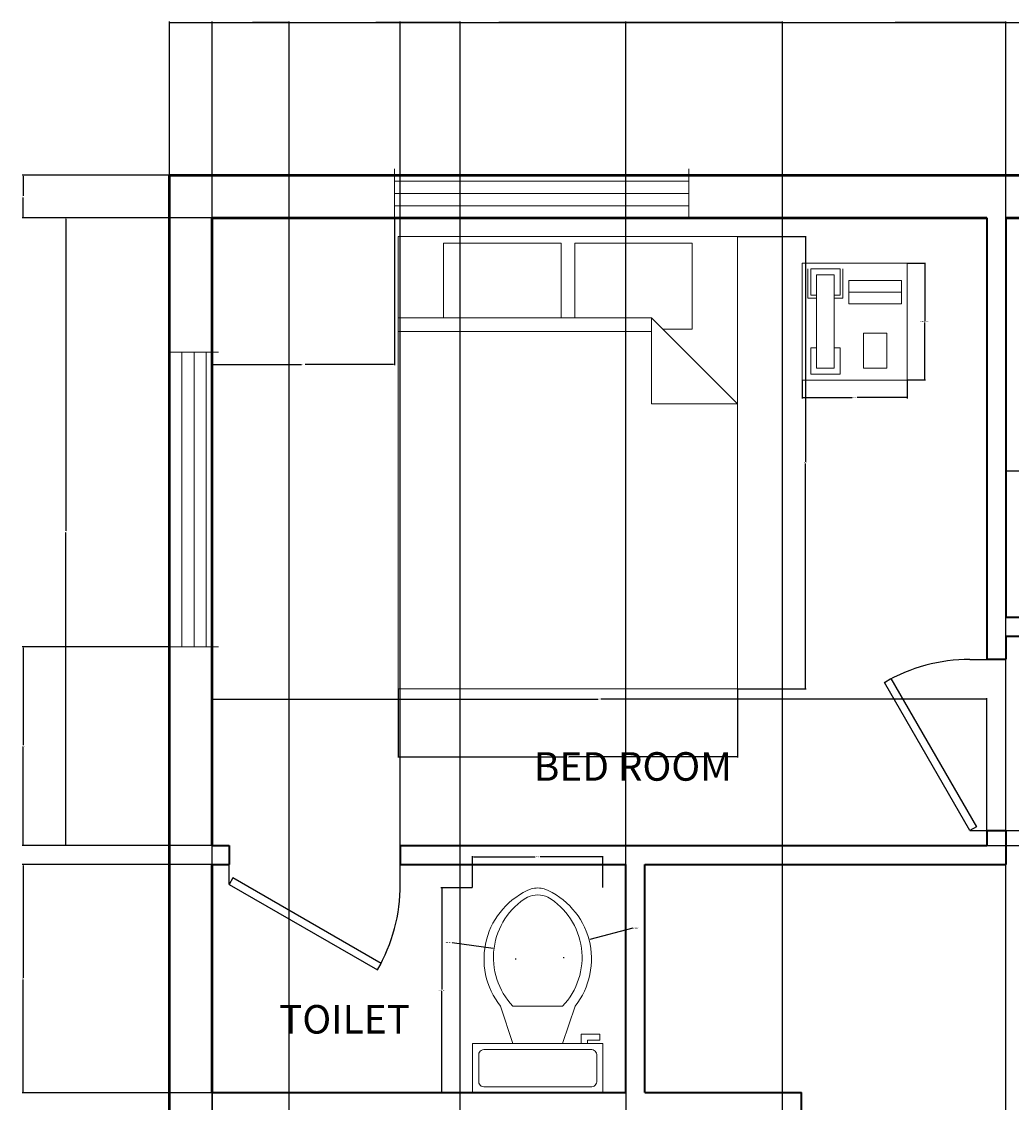
# Model space of a CAD drawing. Units: feet. Extents: x 3746 to 4170, y 1475 to 2148.
# Tile 4 of 5: x 3746 to 3955, y 1920 to 2148. Entities that reach past the tile are written whole.
import ezdxf

# ---------------------------------------------------------------- set-up
doc = ezdxf.new("R2010")
doc.units = ezdxf.units.FT
for name, color, linetype, lineweight in [('A-ANNO-DIMS', 2, 'Continuous', 18), ('A-AREA-IDEN', 7, 'Continuous', 25), ('A-EQPM', 8, 'Continuous', 13), ('A-FLOR-FIXT', 9, 'Continuous', 18), ('A-GLAZ', 91, 'Continuous', 18), ('DOOR', 135, 'Continuous', 25), ('FURNITURE', 43, 'Continuous', 18), ('INWER WALL', 30, 'Continuous', 35), ('OUTER WALL', 31, 'Continuous', 50)]:
    doc.layers.add(name, color=color, linetype=linetype, lineweight=lineweight)
doc.styles.get("Standard").update_dxf_attribs({"font": 'arial.ttf'})
doc.dimstyles.get("Standard").update_dxf_attribs({"dimtxt": 0.18, "dimasz": 0.18, "dimexe": 0.18, "dimexo": 0.0625, "dimgap": 0.09, "dimtad": 0, "dimtih": 1, "dimtoh": 1, "dimdec": 4, "dimzin": 0, "dimdsep": 46, "dimtxsty": 'Standard', "dimcen": 0.09, "dimadec": 0, "dimazin": 0, "dimtfac": 1, "dimtdec": 4, "dimtofl": 0, "dimtmove": 0, "dimatfit": 3, "dimfxl": 1, "dimtolj": 1, "dimtzin": 0, "dimarcsym": 0})

# ---------------------------------------------------------------- blocks, each defined once
blk = doc.blocks.new('*U4')
for p, q in [((0, 0), (0, -6)), ((40, 0), (40, -6))]:
    blk.add_line(p, q)
blk.add_lwpolyline([(0, 0), (34.64, 20), (35.52, 18.48), (0.87, -1.52)], close=True)
blk.add_arc((0, 0), 40, 0, 30)
blk = doc.blocks.new('*U3')
for p, q in [((0, 0), (0, 6)), ((40, 0), (40, 6))]:
    blk.add_line(p, q)
blk.add_lwpolyline([(0, 0), (34.64, -20), (35.52, -18.48), (0.87, 1.52)], close=True)
blk.add_arc((0, 0), 40, 330, 0)
blk = doc.blocks.new('Bed - Queen')
for p, q in [((0, -80.00003), (0, 0)), ((0, 0), (59.99999, 0)), ((59.99999, 0), (59.99999, -80.00003)), ((7.99999, -1.2), (28.79998, -1.2)), ((7.99999, -14.4), (7.99999, -1.2)), ((28.79998, -1.2), (28.79998, -14.4)), ((31.19999, -1.2), (51.99999, -1.2)), ((31.19999, -14.4), (31.19999, -1.2)), ((51.99999, -1.2), (51.99999, -16.4)), ((0, -14.4), (44.8, -14.4)), ((59.99999, -29.6), (44.8, -14.4)), ((44.8, -14.4), (44.8, -29.6)), ((44.8, -16.8), (0, -16.8)), ((51.99999, -16.4), (46.79936, -16.4)), ((44.8, -29.6), (59.99999, -29.6)), ((59.99999, -80.00003), (0, -80.00003))]:
    blk.add_line(p, q)
blk = doc.blocks.new('Toilet - top')
for p, q in [((9.5, -6), (9.5, -2)), ((-10, -8.5), (-8, -8.5)), ((-10, -9.5), (-10, -8.5)), ((-8, -8.5), (-8, -8)), ((-7, -8), (-7, -9.5)), ((-4, -8), (-6, -14)), ((4, -8), (6, -14)), ((-7, -9.5), (-10, -9.5)), ((4, -14), (-4, -14))]:
    blk.add_line(p, q)
blk.add_lwpolyline([(10.5, -8), (10.5, 0), (-10.5, 0), (-10.5, -8)], close=True)
for points in [[(8.5, -1), (-8.5, -1)], [(-9.5, -2), (-9.5, -6)], [(-8.5, -7), (8.5, -7)]]:
    blk.add_lwpolyline(points)
for centre, radius, start, end in [((-8.62, -1.88), 0.884, 81.8699, 188.1301), ((8.62, -1.88), 0.884, 351.8699, 98.1301), ((-8.62, -6.12), 0.884, 171.8699, 278.1301), ((8.62, -6.12), 0.884, 261.8699, 8.1301), ((3.52, -21.58), 12.17, 141.4691, 247.9714), ((4.2, -21.82), 11.33, 136.3677, 238.9468), ((-3.52, -21.58), 12.17, 292.0284, 38.5307), ((-4.2, -21.82), 11.33, 301.053, 43.6321), ((0, -27.88), 4, 245.7318, 294.2682), ((0, -29), 4, 254.8605, 285.1395)]:
    blk.add_arc(centre, radius, start, end)
blk = doc.blocks.new('Phone - Desk')
for p, q in [((-4.5, -5), (-4.5, 5)), ((-4.5, 5), (4.5, 5)), ((4.5, 5), (4.5, -5)), ((-4, 4.5), (-4, 2)), ((-3.75, 4.5), (-3.75, 2.25)), ((-1.25, 4.5), (-3.75, 4.5)), ((-3.25, 4), (-3.25, -4)), ((-3.25, 4), (-1.75, 4)), ((-1.75, -4), (-1.75, 4)), ((-1.25, 2.25), (-1.25, 4.5)), ((-1, 2), (-1, 4.5)), ((4, 3.5), (-0.5, 3.5)), ((-0.5, 3.5), (-0.5, 1.5)), ((4, 1.5), (4, 3.5)), ((-4, 2), (-3.25, 2)), ((-3.75, 2.25), (-3.25, 2.25)), ((-1.75, 2.25), (-1.25, 2.25)), ((-1.75, 2), (-1, 2)), ((-0.5, 2.5), (4, 2.5)), ((-0.5, 1.5), (4, 1.5)), ((2.75, -1), (0.75, -1)), ((0.75, -1), (0.75, -4)), ((2.75, -4), (2.75, -1)), ((-3.75, -2.25), (-3.25, -2.25)), ((-3.75, -4.5), (-3.75, -2.25)), ((-1.75, -2.25), (-1.25, -2.25)), ((-1.25, -2.25), (-1.25, -4.5)), ((-1.25, -4.5), (-3.75, -4.5)), ((-3.25, -4), (-1.75, -4)), ((0.75, -4), (2.75, -4)), ((4.5, -5), (-4.5, -5))]:
    blk.add_line(p, q)
blk = doc.blocks.new('Window - Wood Frame 36 in. Wide plan')
for p, q in [((0, 6), (0, 0)), ((36, 6), (36, 0)), ((0, 4.5), (36, 4.5)), ((0, 3), (36, 3)), ((0, 1.5), (36, 1.5))]:
    blk.add_line(p, q)
blk = doc.blocks.new('*D41')
at = {"layer": 'A-ANNO-DIMS', "color": 0, "lineweight": -2, "transparency": 16777216}
for p, q in [((3897.02, 2102.5), (3911.42, 2102.5)), ((3911.24, 2102.32), (3911.24, 2055.09)), ((3911.24, 2007.5), (3911.24, 2054.73)), ((3897.02, 2007.32), (3911.42, 2007.32))]:
    blk.add_line(p, q, dxfattribs=at)
at = {"layer": 'A-ANNO-DIMS', "color": 0, "transparency": 16777216}
for points in [[(3911.21, 2102.32), (3911.27, 2102.32), (3911.24, 2102.5)], [(3911.21, 2007.5), (3911.27, 2007.5), (3911.24, 2007.32)]]:
    blk.add_solid(points, dxfattribs=at)
at = {"layer": 'Defpoints', "color": 0, "transparency": 16777216}
for p in [(3896.96, 2102.5), (3911.24, 2102.5), (3896.96, 2007.32)]:
    blk.add_point(p, dxfattribs=at)
at = {"layer": 'A-ANNO-DIMS', "color": 0, "transparency": 16777216, "insert": (3911.24, 2054.91), "char_height": 0.18, "attachment_point": 5}
blk.add_mtext('\\A1;BED 95', dxfattribs=at)
blk = doc.blocks.new('*D42')
at = {"layer": 'A-ANNO-DIMS', "color": 0, "lineweight": -2, "transparency": 16777216}
for p, q in [((3825.57, 2007.26), (3825.57, 1992.86)), ((3896.96, 2007.26), (3896.96, 1992.86)), ((3825.75, 1993.04), (3861.06, 1993.04)), ((3896.78, 1993.04), (3861.47, 1993.04))]:
    blk.add_line(p, q, dxfattribs=at)
at = {"layer": 'A-ANNO-DIMS', "color": 0, "transparency": 16777216}
for points in [[(3825.75, 1993.07), (3825.75, 1993.01), (3825.57, 1993.04)], [(3896.78, 1993.07), (3896.78, 1993.01), (3896.96, 1993.04)]]:
    blk.add_solid(points, dxfattribs=at)
at = {"layer": 'Defpoints', "color": 0, "transparency": 16777216}
for p in [(3825.57, 2007.32), (3896.96, 2007.32), (3896.96, 1993.04)]:
    blk.add_point(p, dxfattribs=at)
at = {"layer": 'A-ANNO-DIMS', "color": 0, "transparency": 16777216, "insert": (3861.27, 1993.04), "char_height": 0.18, "attachment_point": 5}
blk.add_mtext('\\A1;71', dxfattribs=at)
blk = doc.blocks.new('*D43')
at = {"layer": 'A-ANNO-DIMS', "color": 0, "lineweight": -2, "transparency": 16777216}
for p, q in [((3841.12, 1965.5), (3834.53, 1965.5)), ((3834.71, 1965.32), (3834.71, 1944.08)), ((3834.71, 1922.47), (3834.71, 1943.71)), ((3841.12, 1922.29), (3834.53, 1922.29))]:
    blk.add_line(p, q, dxfattribs=at)
at = {"layer": 'A-ANNO-DIMS', "color": 0, "transparency": 16777216}
for points in [[(3834.68, 1965.32), (3834.74, 1965.32), (3834.71, 1965.5)], [(3834.68, 1922.47), (3834.74, 1922.47), (3834.71, 1922.29)]]:
    blk.add_solid(points, dxfattribs=at)
at = {"layer": 'Defpoints', "color": 0, "transparency": 16777216}
for p in [(3841.19, 1965.5), (3834.71, 1922.29), (3841.19, 1922.29)]:
    blk.add_point(p, dxfattribs=at)
at = {"layer": 'A-ANNO-DIMS', "color": 0, "transparency": 16777216, "insert": (3834.71, 1943.89), "char_height": 0.18, "attachment_point": 5}
blk.add_mtext('\\A1;WC 43 TYP.', dxfattribs=at)
blk = doc.blocks.new('*D44')
at = {"layer": 'A-ANNO-DIMS', "color": 0, "lineweight": -2, "transparency": 16777216}
for p, q in [((3841.19, 1965.56), (3841.19, 1972.16)), ((3841.37, 1971.98), (3854.39, 1971.98)), ((3868.46, 1971.98), (3855.44, 1971.98)), ((3868.64, 1965.56), (3868.64, 1972.16))]:
    blk.add_line(p, q, dxfattribs=at)
at = {"layer": 'A-ANNO-DIMS', "color": 0, "transparency": 16777216}
for points in [[(3841.37, 1972.01), (3841.37, 1971.95), (3841.19, 1971.98)], [(3868.46, 1972.01), (3868.46, 1971.95), (3868.64, 1971.98)]]:
    blk.add_solid(points, dxfattribs=at)
at = {"layer": 'Defpoints', "color": 0, "transparency": 16777216}
for p in [(3841.19, 1971.98), (3841.19, 1965.5), (3868.64, 1965.5)]:
    blk.add_point(p, dxfattribs=at)
at = {"layer": 'A-ANNO-DIMS', "color": 0, "transparency": 16777216, "insert": (3854.91, 1971.98), "char_height": 0.18, "attachment_point": 5}
blk.add_mtext('\\A1;27 TYP.', dxfattribs=at)
blk = doc.blocks.new('*D45')
at = {"layer": 'A-ANNO-DIMS', "color": 0, "lineweight": -2, "transparency": 16777216}
for p, q in [((3932.72, 2096.9), (3936.53, 2096.9)), ((3936.35, 2096.72), (3936.35, 2084.78)), ((3936.35, 2072.48), (3936.35, 2084.41)), ((3932.72, 2072.3), (3936.53, 2072.3))]:
    blk.add_line(p, q, dxfattribs=at)
at = {"layer": 'A-ANNO-DIMS', "color": 0, "transparency": 16777216}
for points in [[(3936.32, 2096.72), (3936.38, 2096.72), (3936.35, 2096.9)], [(3936.32, 2072.48), (3936.38, 2072.48), (3936.35, 2072.3)]]:
    blk.add_solid(points, dxfattribs=at)
at = {"layer": 'Defpoints', "color": 0, "transparency": 16777216}
for p in [(3932.66, 2096.9), (3936.35, 2096.9), (3932.66, 2072.3)]:
    blk.add_point(p, dxfattribs=at)
at = {"layer": 'A-ANNO-DIMS', "color": 0, "transparency": 16777216, "insert": (3936.35, 2084.6), "char_height": 0.18, "attachment_point": 5}
blk.add_mtext('\\A1;PHONE 25 TYP.', dxfattribs=at)
blk = doc.blocks.new('*D46')
at = {"layer": 'A-ANNO-DIMS', "color": 0, "lineweight": -2, "transparency": 16777216}
for p, q in [((3910.52, 2072.24), (3910.52, 2068.43)), ((3932.66, 2072.24), (3932.66, 2068.43)), ((3910.7, 2068.61), (3921.06, 2068.61)), ((3932.48, 2068.61), (3922.12, 2068.61))]:
    blk.add_line(p, q, dxfattribs=at)
at = {"layer": 'A-ANNO-DIMS', "color": 0, "transparency": 16777216}
for points in [[(3910.7, 2068.64), (3910.7, 2068.58), (3910.52, 2068.61)], [(3932.48, 2068.64), (3932.48, 2068.58), (3932.66, 2068.61)]]:
    blk.add_solid(points, dxfattribs=at)
at = {"layer": 'Defpoints', "color": 0, "transparency": 16777216}
for p in [(3910.52, 2072.3), (3932.66, 2072.3), (3932.66, 2068.61)]:
    blk.add_point(p, dxfattribs=at)
at = {"layer": 'A-ANNO-DIMS', "color": 0, "transparency": 16777216, "insert": (3921.59, 2068.61), "char_height": 0.18, "attachment_point": 5}
blk.add_mtext('\\A1;22 TYP.', dxfattribs=at)
blk = doc.blocks.new('*D55')
at = {"layer": 'A-ANNO-DIMS', "color": 0, "lineweight": -2, "transparency": 16777216}
for p, q in [((3777.43, 2115.45), (3777.43, 2147.69)), ((3777.61, 2147.51), (3957.14, 2147.51)), ((4137.25, 2147.51), (3957.72, 2147.51)), ((4137.43, 2115.45), (4137.43, 2147.69))]:
    blk.add_line(p, q, dxfattribs=at)
at = {"layer": 'A-ANNO-DIMS', "color": 0, "transparency": 16777216}
for points in [[(3777.61, 2147.54), (3777.61, 2147.48), (3777.43, 2147.51)], [(4137.25, 2147.54), (4137.25, 2147.48), (4137.43, 2147.51)]]:
    blk.add_solid(points, dxfattribs=at)
at = {"layer": 'Defpoints', "color": 0, "transparency": 16777216}
for p in [(4137.43, 2147.51), (3777.43, 2115.38), (4137.43, 2115.38)]:
    blk.add_point(p, dxfattribs=at)
at = {"layer": 'A-ANNO-DIMS', "color": 0, "transparency": 16777216, "insert": (3957.43, 2147.51), "char_height": 0.18, "attachment_point": 5}
blk.add_mtext('\\A1;360', dxfattribs=at)
blk = doc.blocks.new('*D57')
at = {"layer": 'A-ANNO-DIMS', "color": 0, "lineweight": -2, "transparency": 16777216}
for p, q in [((3786.43, 1974.45), (3786.43, 2005.36)), ((3949.43, 1974.45), (3949.43, 2005.36)), ((3786.61, 2005.18), (3867.65, 2005.18)), ((3949.25, 2005.18), (3868.21, 2005.18))]:
    blk.add_line(p, q, dxfattribs=at)
at = {"layer": 'A-ANNO-DIMS', "color": 0, "transparency": 16777216}
for points in [[(3786.61, 2005.21), (3786.61, 2005.15), (3786.43, 2005.18)], [(3949.25, 2005.21), (3949.25, 2005.15), (3949.43, 2005.18)]]:
    blk.add_solid(points, dxfattribs=at)
at = {"layer": 'Defpoints', "color": 0, "transparency": 16777216}
for p in [(3949.43, 2005.18), (3786.43, 1974.38), (3949.43, 1974.38)]:
    blk.add_point(p, dxfattribs=at)
at = {"layer": 'A-ANNO-DIMS', "color": 0, "transparency": 16777216, "insert": (3867.93, 2005.18), "char_height": 0.18, "attachment_point": 5}
blk.add_mtext('\\A1;163', dxfattribs=at)
blk = doc.blocks.new('*D58')
at = {"layer": 'A-ANNO-DIMS', "color": 0, "lineweight": -2, "transparency": 16777216}
for p, q in [((3953.43, 2022.45), (3953.43, 2053.36)), ((3953.61, 2053.18), (3977.21, 2053.18)), ((4001.25, 2053.18), (3977.65, 2053.18)), ((4001.43, 2022.45), (4001.43, 2053.36))]:
    blk.add_line(p, q, dxfattribs=at)
at = {"layer": 'A-ANNO-DIMS', "color": 0, "transparency": 16777216}
for points in [[(3953.61, 2053.21), (3953.61, 2053.15), (3953.43, 2053.18)], [(4001.25, 2053.21), (4001.25, 2053.15), (4001.43, 2053.18)]]:
    blk.add_solid(points, dxfattribs=at)
at = {"layer": 'Defpoints', "color": 0, "transparency": 16777216}
for p in [(4001.43, 2053.18), (3953.43, 2022.38), (4001.43, 2022.38)]:
    blk.add_point(p, dxfattribs=at)
at = {"layer": 'A-ANNO-DIMS', "color": 0, "transparency": 16777216, "insert": (3977.43, 2053.18), "char_height": 0.18, "attachment_point": 5}
blk.add_mtext('\\A1;48', dxfattribs=at)
blk = doc.blocks.new('*D60')
at = {"layer": 'A-ANNO-DIMS', "color": 0, "lineweight": -2, "transparency": 16777216}
for p, q in [((3786.37, 2106.38), (3755.45, 2106.38)), ((3755.63, 2106.2), (3755.63, 2040.56)), ((3755.63, 1974.56), (3755.63, 2040.2)), ((3786.37, 1974.38), (3755.45, 1974.38))]:
    blk.add_line(p, q, dxfattribs=at)
at = {"layer": 'A-ANNO-DIMS', "color": 0, "transparency": 16777216}
for points in [[(3755.6, 2106.2), (3755.66, 2106.2), (3755.63, 2106.38)], [(3755.6, 1974.56), (3755.66, 1974.56), (3755.63, 1974.38)]]:
    blk.add_solid(points, dxfattribs=at)
at = {"layer": 'Defpoints', "color": 0, "transparency": 16777216}
for p in [(3755.63, 2106.38), (3786.43, 2106.38), (3786.43, 1974.38)]:
    blk.add_point(p, dxfattribs=at)
at = {"layer": 'A-ANNO-DIMS', "color": 0, "transparency": 16777216, "insert": (3755.63, 2040.38), "char_height": 0.18, "attachment_point": 5}
blk.add_mtext('\\A1;132', dxfattribs=at)
blk = doc.blocks.new('*D62')
at = {"layer": 'A-ANNO-DIMS', "color": 0, "lineweight": -2, "transparency": 16777216}
for p, q in [((3786.37, 1970.38), (3746.45, 1970.38)), ((3746.63, 1970.2), (3746.63, 1946.56)), ((3746.63, 1922.56), (3746.63, 1946.2)), ((3786.37, 1922.38), (3746.45, 1922.38))]:
    blk.add_line(p, q, dxfattribs=at)
at = {"layer": 'A-ANNO-DIMS', "color": 0, "transparency": 16777216}
for points in [[(3746.6, 1970.2), (3746.66, 1970.2), (3746.63, 1970.38)], [(3746.6, 1922.56), (3746.66, 1922.56), (3746.63, 1922.38)]]:
    blk.add_solid(points, dxfattribs=at)
at = {"layer": 'Defpoints', "color": 0, "transparency": 16777216}
for p in [(3786.43, 1970.38), (3746.63, 1922.38), (3786.43, 1922.38)]:
    blk.add_point(p, dxfattribs=at)
at = {"layer": 'A-ANNO-DIMS', "color": 0, "transparency": 16777216, "insert": (3746.63, 1946.38), "char_height": 0.18, "attachment_point": 5}
blk.add_mtext('\\A1;48', dxfattribs=at)
blk = doc.blocks.new('*D63')
at = {"layer": 'A-ANNO-DIMS', "color": 0, "lineweight": -2, "transparency": 16777216}
for p, q in [((3786.43, 1970.32), (3786.43, 1474.8)), ((3873.43, 1922.32), (3873.43, 1474.8)), ((3786.61, 1474.98), (3829.71, 1474.98)), ((3873.25, 1474.98), (3830.15, 1474.98))]:
    blk.add_line(p, q, dxfattribs=at)
at = {"layer": 'A-ANNO-DIMS', "color": 0, "transparency": 16777216}
for points in [[(3786.61, 1475.01), (3786.61, 1474.95), (3786.43, 1474.98)], [(3873.25, 1475.01), (3873.25, 1474.95), (3873.43, 1474.98)]]:
    blk.add_solid(points, dxfattribs=at)
at = {"layer": 'Defpoints', "color": 0, "transparency": 16777216}
for p in [(3786.43, 1970.38), (3873.43, 1922.38), (3873.43, 1474.98)]:
    blk.add_point(p, dxfattribs=at)
at = {"layer": 'A-ANNO-DIMS', "color": 0, "transparency": 16777216, "insert": (3829.93, 1474.98), "char_height": 0.18, "attachment_point": 5}
blk.add_mtext('\\A1;87', dxfattribs=at)
blk = doc.blocks.new('*D64')
at = {"layer": 'A-ANNO-DIMS', "color": 0, "lineweight": -2, "transparency": 16777216}
for p, q in [((3826, 1970.45), (3826, 2147.69)), ((3826.18, 2147.51), (3849.31, 2147.51)), ((3873.25, 2147.51), (3850.11, 2147.51)), ((3873.43, 1970.45), (3873.43, 2147.69))]:
    blk.add_line(p, q, dxfattribs=at)
at = {"layer": 'A-ANNO-DIMS', "color": 0, "transparency": 16777216}
for points in [[(3826.18, 2147.54), (3826.18, 2147.48), (3826, 2147.51)], [(3873.25, 2147.54), (3873.25, 2147.48), (3873.43, 2147.51)]]:
    blk.add_solid(points, dxfattribs=at)
at = {"layer": 'Defpoints', "color": 0, "transparency": 16777216}
for p in [(3873.43, 2147.51), (3826, 1970.38), (3873.43, 1970.38)]:
    blk.add_point(p, dxfattribs=at)
at = {"layer": 'A-ANNO-DIMS', "color": 0, "transparency": 16777216, "insert": (3849.71, 2147.51), "char_height": 0.18, "attachment_point": 5}
blk.add_mtext('\\A1;47.43', dxfattribs=at)
blk = doc.blocks.new('*D66')
at = {"layer": 'A-ANNO-DIMS', "color": 0, "lineweight": -2, "transparency": 16777216}
for p, q in [((3786.43, 1918.45), (3786.43, 2147.69)), ((3786.61, 2147.51), (3846.15, 2147.51)), ((3906.25, 2147.51), (3846.71, 2147.51)), ((3906.43, 1918.45), (3906.43, 2147.69))]:
    blk.add_line(p, q, dxfattribs=at)
at = {"layer": 'A-ANNO-DIMS', "color": 0, "transparency": 16777216}
for points in [[(3786.61, 2147.54), (3786.61, 2147.48), (3786.43, 2147.51)], [(3906.25, 2147.54), (3906.25, 2147.48), (3906.43, 2147.51)]]:
    blk.add_solid(points, dxfattribs=at)
at = {"layer": 'Defpoints', "color": 0, "transparency": 16777216}
for p in [(3906.43, 2147.51), (3786.43, 1918.38), (3906.43, 1918.38)]:
    blk.add_point(p, dxfattribs=at)
at = {"layer": 'A-ANNO-DIMS', "color": 0, "transparency": 16777216, "insert": (3846.43, 2147.51), "char_height": 0.18, "attachment_point": 5}
blk.add_mtext('\\A1;120', dxfattribs=at)
blk = doc.blocks.new('*D69')
at = {"layer": 'A-ANNO-DIMS', "color": 0, "lineweight": -2, "transparency": 16777216}
for p, q in [((3802.61, 1835.45), (3802.61, 2147.69)), ((3802.79, 2147.51), (3820.39, 2147.51)), ((3838.43, 2147.51), (3820.83, 2147.51)), ((3838.61, 1835.45), (3838.61, 2147.69))]:
    blk.add_line(p, q, dxfattribs=at)
at = {"layer": 'A-ANNO-DIMS', "color": 0, "transparency": 16777216}
for points in [[(3802.79, 2147.54), (3802.79, 2147.48), (3802.61, 2147.51)], [(3838.43, 2147.54), (3838.43, 2147.48), (3838.61, 2147.51)]]:
    blk.add_solid(points, dxfattribs=at)
at = {"layer": 'Defpoints', "color": 0, "transparency": 16777216}
for p in [(3838.61, 2147.51), (3802.61, 1835.38), (3838.61, 1835.38)]:
    blk.add_point(p, dxfattribs=at)
at = {"layer": 'A-ANNO-DIMS', "color": 0, "transparency": 16777216, "insert": (3820.61, 2147.51), "char_height": 0.18, "attachment_point": 5}
blk.add_mtext('\\A1;36', dxfattribs=at)
blk = doc.blocks.new('*D70')
at = {"layer": 'A-ANNO-DIMS', "color": 0, "lineweight": -2, "transparency": 16777216}
for p, q in [((3786.43, 1839.45), (3786.43, 2147.69)), ((3786.61, 2147.51), (3794.13, 2147.51)), ((3802.43, 2147.51), (3794.9, 2147.51)), ((3802.61, 1839.45), (3802.61, 2147.69))]:
    blk.add_line(p, q, dxfattribs=at)
at = {"layer": 'A-ANNO-DIMS', "color": 0, "transparency": 16777216}
for points in [[(3786.61, 2147.54), (3786.61, 2147.48), (3786.43, 2147.51)], [(3802.43, 2147.54), (3802.43, 2147.48), (3802.61, 2147.51)]]:
    blk.add_solid(points, dxfattribs=at)
at = {"layer": 'Defpoints', "color": 0, "transparency": 16777216}
for p in [(3802.61, 2147.51), (3786.43, 1839.38), (3802.61, 1839.38)]:
    blk.add_point(p, dxfattribs=at)
at = {"layer": 'A-ANNO-DIMS', "color": 0, "transparency": 16777216, "insert": (3794.52, 2147.51), "char_height": 0.18, "attachment_point": 5}
blk.add_mtext('\\A1;16.18', dxfattribs=at)
blk = doc.blocks.new('*D77')
at = {"layer": 'A-ANNO-DIMS', "color": 0, "lineweight": -2, "transparency": 16777216}
for p, q in [((3953.43, 1839.45), (3953.43, 2147.69)), ((3953.61, 2147.51), (3977.21, 2147.51)), ((4001.25, 2147.51), (3977.65, 2147.51)), ((4001.43, 1839.45), (4001.43, 2147.69))]:
    blk.add_line(p, q, dxfattribs=at)
at = {"layer": 'A-ANNO-DIMS', "color": 0, "transparency": 16777216}
for points in [[(3953.61, 2147.54), (3953.61, 2147.48), (3953.43, 2147.51)], [(4001.25, 2147.54), (4001.25, 2147.48), (4001.43, 2147.51)]]:
    blk.add_solid(points, dxfattribs=at)
at = {"layer": 'Defpoints', "color": 0, "transparency": 16777216}
for p in [(4001.43, 2147.51), (3953.43, 1839.38), (4001.43, 1839.38)]:
    blk.add_point(p, dxfattribs=at)
at = {"layer": 'A-ANNO-DIMS', "color": 0, "transparency": 16777216, "insert": (3977.43, 2147.51), "char_height": 0.18, "attachment_point": 5}
blk.add_mtext('\\A1;48', dxfattribs=at)
blk = doc.blocks.new('*D78')
at = {"layer": 'A-ANNO-DIMS', "color": 0, "lineweight": -2, "transparency": 16777216}
for p, q in [((3906.43, 1835.45), (3906.43, 2147.69)), ((3906.61, 2147.51), (3929.71, 2147.51)), ((3953.25, 2147.51), (3930.15, 2147.51)), ((3953.43, 1835.45), (3953.43, 2147.69))]:
    blk.add_line(p, q, dxfattribs=at)
at = {"layer": 'A-ANNO-DIMS', "color": 0, "transparency": 16777216}
for points in [[(3906.61, 2147.54), (3906.61, 2147.48), (3906.43, 2147.51)], [(3953.25, 2147.54), (3953.25, 2147.48), (3953.43, 2147.51)]]:
    blk.add_solid(points, dxfattribs=at)
at = {"layer": 'Defpoints', "color": 0, "transparency": 16777216}
for p in [(3953.43, 2147.51), (3906.43, 1835.38), (3953.43, 1835.38)]:
    blk.add_point(p, dxfattribs=at)
at = {"layer": 'A-ANNO-DIMS', "color": 0, "transparency": 16777216, "insert": (3929.93, 2147.51), "char_height": 0.18, "attachment_point": 5}
blk.add_mtext('\\A1;47', dxfattribs=at)
blk = doc.blocks.new('*D79')
at = {"layer": 'A-ANNO-DIMS', "color": 0, "lineweight": -2, "transparency": 16777216}
for p, q in [((3777.37, 2115.38), (3746.45, 2115.38)), ((3746.63, 2115.2), (3746.63, 2111.06)), ((3746.63, 2106.56), (3746.63, 2110.7)), ((3786.37, 2106.38), (3746.45, 2106.38))]:
    blk.add_line(p, q, dxfattribs=at)
at = {"layer": 'A-ANNO-DIMS', "color": 0, "transparency": 16777216}
for points in [[(3746.6, 2115.2), (3746.66, 2115.2), (3746.63, 2115.38)], [(3746.6, 2106.56), (3746.66, 2106.56), (3746.63, 2106.38)]]:
    blk.add_solid(points, dxfattribs=at)
at = {"layer": 'Defpoints', "color": 0, "transparency": 16777216}
for p in [(3777.43, 2115.38), (3746.63, 2106.38), (3786.43, 2106.38)]:
    blk.add_point(p, dxfattribs=at)
at = {"layer": 'A-ANNO-DIMS', "color": 0, "transparency": 16777216, "insert": (3746.63, 2110.88), "char_height": 0.18, "attachment_point": 5}
blk.add_mtext('\\A1;9', dxfattribs=at)
blk = doc.blocks.new('*D80')
at = {"layer": 'A-ANNO-DIMS', "color": 0, "lineweight": -2, "transparency": 16777216}
for p, q in [((3786.43, 2106.32), (3786.43, 2075.4)), ((3824.76, 2106.32), (3824.76, 2075.4)), ((3786.61, 2075.58), (3805.2, 2075.58)), ((3824.58, 2075.58), (3805.99, 2075.58))]:
    blk.add_line(p, q, dxfattribs=at)
at = {"layer": 'A-ANNO-DIMS', "color": 0, "transparency": 16777216}
for points in [[(3786.61, 2075.61), (3786.61, 2075.55), (3786.43, 2075.58)], [(3824.58, 2075.61), (3824.58, 2075.55), (3824.76, 2075.58)]]:
    blk.add_solid(points, dxfattribs=at)
at = {"layer": 'Defpoints', "color": 0, "transparency": 16777216}
for p in [(3786.43, 2106.38), (3824.76, 2106.38), (3786.43, 2075.58)]:
    blk.add_point(p, dxfattribs=at)
at = {"layer": 'A-ANNO-DIMS', "color": 0, "transparency": 16777216, "insert": (3805.59, 2075.58), "char_height": 0.18, "attachment_point": 5}
blk.add_mtext('\\A1;38.33', dxfattribs=at)
blk = doc.blocks.new('*D82')
at = {"layer": 'A-ANNO-DIMS', "color": 0, "lineweight": -2, "transparency": 16777216}
for p, q in [((3777.37, 2016.17), (3746.45, 2016.17)), ((3746.63, 2015.99), (3746.63, 1995.46)), ((3746.63, 1974.56), (3746.63, 1995.1)), ((3786.37, 1974.38), (3746.45, 1974.38))]:
    blk.add_line(p, q, dxfattribs=at)
at = {"layer": 'A-ANNO-DIMS', "color": 0, "transparency": 16777216}
for points in [[(3746.6, 2015.99), (3746.66, 2015.99), (3746.63, 2016.17)], [(3746.6, 1974.56), (3746.66, 1974.56), (3746.63, 1974.38)]]:
    blk.add_solid(points, dxfattribs=at)
at = {"layer": 'Defpoints', "color": 0, "transparency": 16777216}
for p in [(3746.63, 2016.17), (3777.43, 2016.17), (3786.43, 1974.38)]:
    blk.add_point(p, dxfattribs=at)
at = {"layer": 'A-ANNO-DIMS', "color": 0, "transparency": 16777216, "insert": (3746.63, 1995.28), "char_height": 0.18, "attachment_point": 5}
blk.add_mtext('\\A1;41.79', dxfattribs=at)
blk = doc.blocks.new('*D90')
at = {"layer": 'A-ANNO-DIMS', "color": 0, "lineweight": -2, "transparency": 16777216}
for p, q in [((3949.49, 1977.56), (3980.41, 1977.56)), ((3980.23, 1977.38), (3980.23, 1976.15)), ((3980.23, 1974.56), (3980.23, 1975.79)), ((3949.49, 1974.38), (3980.41, 1974.38))]:
    blk.add_line(p, q, dxfattribs=at)
at = {"layer": 'A-ANNO-DIMS', "color": 0, "transparency": 16777216}
for points in [[(3980.2, 1977.38), (3980.26, 1977.38), (3980.23, 1977.56)], [(3980.2, 1974.56), (3980.26, 1974.56), (3980.23, 1974.38)]]:
    blk.add_solid(points, dxfattribs=at)
at = {"layer": 'Defpoints', "color": 0, "transparency": 16777216}
for p in [(3949.43, 1977.56), (3949.43, 1974.38), (3980.23, 1974.38)]:
    blk.add_point(p, dxfattribs=at)
at = {"layer": 'A-ANNO-DIMS', "color": 0, "transparency": 16777216, "insert": (3980.23, 1975.97), "char_height": 0.18, "attachment_point": 5}
blk.add_mtext('\\A1;3.18', dxfattribs=at)
blk = doc.blocks.new('*D93')
at = {"layer": 'A-ANNO-DIMS', "color": 0, "lineweight": -2, "transparency": 16777216}
for p, q in [((3874.93, 1956.98), (3865.88, 1954.6)), ((3850.22, 1950.51), (3850.4, 1950.51)), ((3850.31, 1950.42), (3850.31, 1950.6))]:
    blk.add_line(p, q, dxfattribs=at)
at = {"layer": 'A-ANNO-DIMS', "color": 0, "transparency": 16777216}
blk.add_solid([(3865.87, 1954.62), (3865.88, 1954.57), (3865.7, 1954.55)], dxfattribs=at)
at = {"layer": 'Defpoints', "color": 0, "transparency": 16777216}
for p in [(3865.7, 1954.55), (3850.31, 1950.51)]:
    blk.add_point(p, dxfattribs=at)
at = {"layer": 'A-ANNO-DIMS', "color": 0, "transparency": 16777216, "insert": (3875.59, 1956.98), "char_height": 0.18, "attachment_point": 5}
blk.add_mtext('\\A1;4X R15.91', dxfattribs=at)
blk = doc.blocks.new('*D94')
at = {"layer": 'A-ANNO-DIMS', "color": 0, "lineweight": -2, "transparency": 16777216}
for p, q in [((3836.92, 1953.97), (3845.55, 1952.81)), ((3860.32, 1950.82), (3860.5, 1950.82)), ((3860.41, 1950.73), (3860.41, 1950.91))]:
    blk.add_line(p, q, dxfattribs=at)
at = {"layer": 'A-ANNO-DIMS', "color": 0, "transparency": 16777216}
blk.add_solid([(3845.55, 1952.84), (3845.54, 1952.78), (3845.73, 1952.79)], dxfattribs=at)
at = {"layer": 'Defpoints', "color": 0, "transparency": 16777216}
for p in [(3845.73, 1952.79), (3860.41, 1950.82)]:
    blk.add_point(p, dxfattribs=at)
at = {"layer": 'A-ANNO-DIMS', "color": 0, "transparency": 16777216, "insert": (3836.17, 1953.97), "char_height": 0.18, "attachment_point": 5}
blk.add_mtext('\\A1;4X R14.813', dxfattribs=at)

msp = doc.modelspace()

# ---------------------------------------------------------------- linework, layer by layer
at = {"layer": 'INWER WALL'}
for p, q in [((3949.4289, 2106.3828), (3949.4289, 2013.5622)), ((3953.4289, 2106.3828), (3953.4289, 2022.3828)), ((3953.4289, 2022.3828), (4001.4289, 2022.3828)), ((3953.4289, 2018.3828), (4001.4289, 2018.3828)), ((3953.4289, 2018.3828), (3953.4289, 2013.5622)), ((3949.4289, 2013.5622), (3953.4289, 2013.5622)), ((3949.4289, 1977.5622), (3953.4289, 1977.5622)), ((3949.4289, 1977.5622), (3949.4289, 1974.3828)), ((3953.4289, 1977.5622), (3953.4289, 1970.3828)), ((3786.4289, 1974.3828), (3789.9958, 1974.3828)), ((3789.9958, 1974.3828), (3789.9958, 1970.3828)), ((3825.9958, 1974.3828), (3825.9958, 1970.3828)), ((3825.9958, 1974.3828), (3949.4289, 1974.3828)), ((3786.4289, 1970.3828), (3789.9958, 1970.3828)), ((3825.9958, 1970.3828), (3873.4289, 1970.3828)), ((3825.9958, 1970.3828), (3873.4289, 1970.3828)), ((3873.4289, 1922.3828), (3873.4289, 1970.3828)), ((3877.4289, 1922.3828), (3877.4289, 1970.3828)), ((3877.4289, 1970.3828), (3953.4289, 1970.3828)), ((3786.4289, 1922.3828), (3873.4289, 1922.3828)), ((3877.4289, 1922.3828), (3910.4289, 1922.3828)), ((3910.4289, 1892.8248), (3910.4289, 1922.3828))]:
    msp.add_line(p, q, dxfattribs=at)
at = {"layer": 'OUTER WALL'}
for p, q in [((3786.4289, 2106.3828), (3949.4289, 2106.3828)), ((3786.4289, 1974.3828), (3786.4289, 2106.3828)), ((3953.4289, 2106.3828), (4001.4289, 2106.3828)), ((3786.4289, 1922.3828), (3786.4289, 1970.3828))]:
    msp.add_line(p, q, dxfattribs=at)
msp.add_lwpolyline([(3948.7526, 1635.3828), (3777.4289, 1635.3828), (3777.4289, 2115.3828), (4137.4289, 2115.3828), (4137.4289, 1635.3828), (4068.7526, 1635.3828)], dxfattribs=at)

# ---------------------------------------------------------------- block references
at = {"layer": 'A-EQPM', "xscale": 2.45986272692771, "yscale": 2.45986272692771, "zscale": 2.45986272692771}
msp.add_blockref('Phone - Desk', (3921.5888, 2084.598), dxfattribs=at)
at = {"layer": 'A-FLOR-FIXT', "xscale": 1.307475105199699, "yscale": 1.307475105199699, "zscale": 1.307475105199699, "rotation": 180}
msp.add_blockref('Toilet - top', (3854.9149, 1922.2908), dxfattribs=at)
at = {"layer": 'A-GLAZ', "xscale": 1.721338572628536, "yscale": 1.721338572628536, "zscale": 1.721338572628536}
msp.add_blockref('Window - Wood Frame 36 in. Wide plan', (3824.758, 2106.3828), dxfattribs=at)
at = {"layer": 'A-GLAZ', "xscale": 1.721338572628536, "yscale": 1.721338572628536, "zscale": 1.721338572628536, "rotation": 90}
msp.add_blockref('Window - Wood Frame 36 in. Wide plan', (3787.7569, 2016.1747), dxfattribs=at)
at = {"layer": 'DOOR', "xscale": 0.9000000000000054, "yscale": 0.9000000000000054, "zscale": 0.9000000000000054, "rotation": 90}
msp.add_blockref('*U4', (3945.8507, 1977.5091), dxfattribs=at)
at = {"layer": 'DOOR', "xscale": 0.9000000000000054, "yscale": 0.9000000000000054, "zscale": 0.9000000000000054}
msp.add_blockref('*U3', (3789.9958, 1966.1994), dxfattribs=at)
at = {"layer": 'FURNITURE', "xscale": 1.189767569118021, "yscale": 1.189767569118021, "zscale": 1.189767569118021}
msp.add_blockref('Bed - Queen', (3825.5721, 2102.5011), dxfattribs=at)

# ---------------------------------------------------------------- texts
at = {"layer": 'A-AREA-IDEN', "char_height": 6, "attachment_point": 1}
for s, insert in [('\\pxt8;BED ROOM', (3854.0865, 1994.006)), ('TOILET', (3800.487, 1940.8128))]:
    msp.add_mtext_dynamic_manual_height_columns(s, width=45.721785, gutter_width=12.5, heights=[0], dxfattribs=dict(at, insert=insert))

# ---------------------------------------------------------------- dimensions: what is measured, and where the dimension line sits
at = {"layer": 'A-ANNO-DIMS'}
for base, p1, p2, override, picture, middle in [((4137.4289, 2147.5109), (3777.4289, 2115.3828), (4137.4289, 2115.3828), {"dimdec": 0, "dimlfac": 1, "dimrnd": 0, "dimzin": 0, "dimdsep": 46, "dimlunit": 2}, '*D55', (3957.4289, 2147.5109)), ((3906.4289, 2147.5109), (3786.4289, 1918.3828), (3906.4289, 1918.3828), {"dimdec": 0, "dimlfac": 1, "dimrnd": 0, "dimzin": 0, "dimdsep": 46, "dimlunit": 2}, '*D66', (3846.4289, 2147.5109)), ((3802.6077, 2147.5109), (3786.4289, 1839.3828), (3802.6077, 1839.3828), {"dimdec": 2, "dimlfac": 1, "dimrnd": 0, "dimzin": 0, "dimdsep": 46, "dimlunit": 2}, '*D70', (3794.5183, 2147.5109)), ((3838.6077, 2147.5109), (3802.6077, 1835.3828), (3838.6077, 1835.3828), {"dimdec": 0, "dimlfac": 1, "dimrnd": 0, "dimzin": 0, "dimdsep": 46, "dimlunit": 2}, '*D69', (3820.6077, 2147.5109)), ((3873.4289, 2147.5109), (3825.9958, 1970.3828), (3873.4289, 1970.3828), {"dimdec": 2, "dimlfac": 1, "dimrnd": 0, "dimzin": 0, "dimdsep": 46, "dimlunit": 2}, '*D64', (3849.7123, 2147.5109)), ((3953.4289, 2147.5109), (3906.4289, 1835.3828), (3953.4289, 1835.3828), {"dimdec": 0, "dimlfac": 1, "dimrnd": 0, "dimzin": 0, "dimdsep": 46, "dimlunit": 2}, '*D78', (3929.9289, 2147.5109)), ((4001.4289, 2147.5109), (3953.4289, 1839.3828), (4001.4289, 1839.3828), {"dimdec": 0, "dimlfac": 1, "dimrnd": 0, "dimzin": 0, "dimdsep": 46, "dimlunit": 2}, '*D77', (3977.4289, 2147.5109)), ((4001.4289, 2053.1828), (3953.4289, 2022.3828), (4001.4289, 2022.3828), {"dimdec": 0, "dimlfac": 1, "dimrnd": 0, "dimzin": 0, "dimdsep": 46, "dimlunit": 2}, '*D58', (3977.4289, 2053.1828)), ((3949.4289, 2005.1828), (3786.4289, 1974.3828), (3949.4289, 1974.3828), {"dimdec": 0, "dimlfac": 1, "dimrnd": 0, "dimzin": 0, "dimdsep": 46, "dimlunit": 2}, '*D57', (3867.9289, 2005.1828)), ((3896.9581, 1993.0424), (3825.5721, 2007.3196), (3896.9581, 2007.3196), {"dimdec": 0, "dimlfac": 1, "dimrnd": 0, "dimzin": 0, "dimdsep": 46, "dimlunit": 2}, '*D42', (3861.2651, 1993.0424)), ((3873.4289, 1474.98), (3786.4289, 1970.3828), (3873.4289, 1922.3828), {"dimdec": 0, "dimlfac": 1, "dimrnd": 0, "dimzin": 0, "dimdsep": 46, "dimlunit": 2}, '*D63', (3829.9289, 1474.98))]:
    dim = msp.add_linear_dim(base=base, p1=p1, p2=p2, dimstyle='Standard', override=override, dxfattribs=at)
    dim.commit()
    dim.dimension.update_dxf_attribs({"geometry": picture, "text_midpoint": middle})
for base, p1, p2, angle, override, picture, middle in [((3746.6289, 2106.3828), (3777.4289, 2115.3828), (3786.4289, 2106.3828), 90, {"dimdec": 0, "dimlfac": 1, "dimrnd": 0, "dimzin": 0, "dimdsep": 46, "dimlunit": 2}, '*D79', (3746.6289, 2110.8828)), ((3755.6289, 2106.3828), (3786.4289, 1974.3828), (3786.4289, 2106.3828), 90, {"dimdec": 0, "dimlfac": 1, "dimrnd": 0, "dimzin": 0, "dimdsep": 46, "dimlunit": 2}, '*D60', (3755.6289, 2040.3828)), ((3786.4289, 2075.5828), (3824.758, 2106.3828), (3786.4289, 2106.3828), 180, {"dimdec": 2, "dimlfac": 1, "dimrnd": 0, "dimzin": 0, "dimdsep": 46, "dimlunit": 2}, '*D80', (3805.5934, 2075.5828)), ((3746.6289, 2016.1747), (3786.4289, 1974.3828), (3777.4289, 2016.1747), 90, {"dimdec": 2, "dimlfac": 1, "dimrnd": 0, "dimzin": 0, "dimdsep": 46, "dimlunit": 2}, '*D82', (3746.6289, 1995.2788)), ((3980.2289, 1974.3828), (3949.4289, 1977.5622), (3949.4289, 1974.3828), 270, {"dimdec": 2, "dimlfac": 1, "dimrnd": 0, "dimzin": 0, "dimdsep": 46, "dimlunit": 2}, '*D90', (3980.2289, 1975.9725)), ((3746.6289, 1922.3828), (3786.4289, 1970.3828), (3786.4289, 1922.3828), 90, {"dimdec": 0, "dimlfac": 1, "dimrnd": 0, "dimzin": 0, "dimdsep": 46, "dimlunit": 2}, '*D62', (3746.6289, 1946.3828))]:
    dim = msp.add_linear_dim(base=base, p1=p1, p2=p2, angle=angle, dimstyle='Standard', override=override, dxfattribs=at)
    dim.commit()
    dim.dimension.update_dxf_attribs({"geometry": picture, "text_midpoint": middle})
for base, p1, p2, angle, text, picture, middle in [((3911.2353, 2102.5011), (3896.9581, 2007.3196), (3896.9581, 2102.5011), 90, 'BED <>', '*D41', (3911.2353, 2054.9104)), ((3936.3479, 2096.8973), (3932.6582, 2072.2986), (3932.6582, 2096.8973), 90, 'PHONE <> TYP.', '*D45', (3936.3479, 2084.598)), ((3841.1864, 1971.979), (3868.6434, 1965.4979), (3841.1864, 1965.4979), 180, '<> TYP.', '*D44', (3854.9149, 1971.979)), ((3834.7054, 1922.2908), (3841.1864, 1965.4979), (3841.1864, 1922.2908), 270, 'WC <> TYP.', '*D43', (3834.7054, 1943.8943))]:
    dim = msp.add_linear_dim(base=base, p1=p1, p2=p2, angle=angle, text=text, dimstyle='Standard', override={"dimdec": 0, "dimlfac": 1, "dimrnd": 0, "dimzin": 0, "dimdsep": 46, "dimlunit": 2}, dxfattribs=at)
    dim.commit()
    dim.dimension.update_dxf_attribs({"geometry": picture, "text_midpoint": middle})
dim = msp.add_linear_dim(base=(3932.6582, 2068.6088), p1=(3910.5194, 2072.2986), p2=(3932.6582, 2072.2986), text='<> TYP.', dimstyle='Standard', override={"dimdec": 0, "dimlfac": 1, "dimrnd": 0, "dimzin": 0, "dimdsep": 46, "dimlunit": 2}, dxfattribs=at)
dim.commit()
dim.dimension.update_dxf_attribs({"geometry": '*D46', "text_midpoint": (3921.5888, 2068.6088)})
for center, mpoint, override, picture, middle in [((3850.3132, 1950.5067), (3865.7016, 1954.5499), {"dimdec": 2, "dimlfac": 1, "dimrnd": 0, "dimzin": 0, "dimdsep": 46, "dimlunit": 2}, '*D93', (3874.9346, 1956.9758)), ((3860.4062, 1950.8165), (3845.7256, 1952.7901), {"dimdec": 3, "dimlfac": 1, "dimrnd": 0, "dimzin": 0, "dimdsep": 46, "dimlunit": 2}, '*D94', (3836.9173, 1953.9742))]:
    dim = msp.add_radius_dim(center=center, mpoint=mpoint, text='4X <>', dimstyle='Standard', override=override, dxfattribs=at)
    dim.commit()
    dim.dimension.update_dxf_attribs({"geometry": picture, "text_midpoint": middle, "dimtype": 164})

doc.saveas('drawing.dxf')
